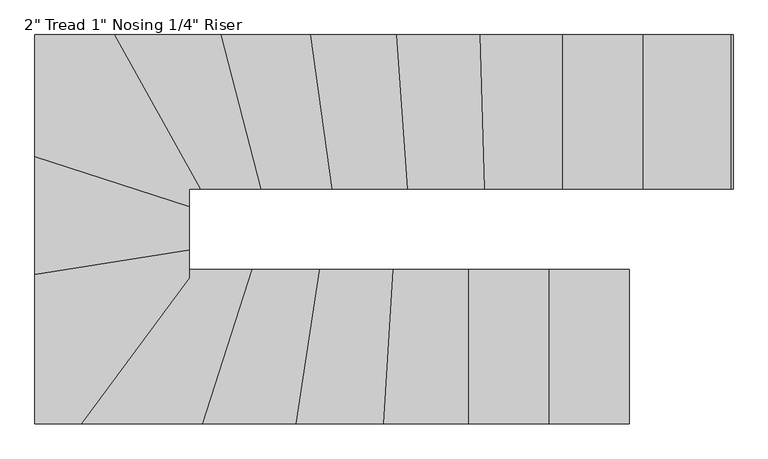
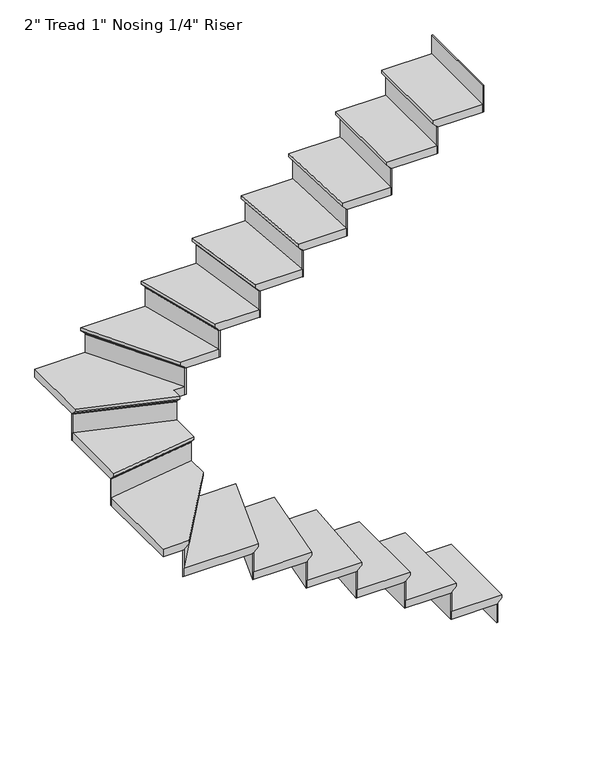
"""IFC4 building model written with IfcOpenShell, lengths in millimetres: stair flight geometry."""

from ifc_helpers import new_model, si_unit, origin, place, context, project, spatial, faceted_brep, source, transform, mapped, element, save


def stair_flight_19b8669d(model_context):
    return source(origin(), model_context, "Body", "Brep", [
        faceted_brep([(-264.8831579, 264.4433073, 9751.4833333), (-264.8831579, 264.4433073, 9770.5333333), (-264.8831579, -271.8029286, 9770.5333333), (-264.8831579, -271.8029286, 9751.4833333), (-290.2831579, 264.4433073, 9726.0833333), (-290.2831579, -271.8029286, 9726.0833333), (-569.6831579, 264.4433073, 9770.5333333), (-569.6831579, -271.8029286, 9770.5333333), (-290.2831579, -271.8029286, 9719.7333333), (-569.6831579, -271.8029286, 9719.7333333), (-569.6831579, 264.4433073, 9719.7333333), (-290.2831579, 264.4433073, 9719.7333333)], [[[0, 1, 2, 3]], [[4, 0, 3, 5]], [[2, 1, 6, 7]], [[8, 9, 10, 11]], [[2, 7, 9, 8, 5, 3]], [[8, 11, 4, 5]], [[6, 1, 0, 4, 11, 10]], [[7, 6, 10, 9]]]),
        faceted_brep([(-290.2831579, 264.4433073, 9719.7333333), (-290.2831579, 264.4433073, 9601.2), (-296.6331579, 264.4433073, 9601.2), (-296.6331579, 264.4433073, 9719.7333333), (-290.2831579, -271.8029286, 9719.7333333), (-296.6331579, -271.8029286, 9719.7333333), (-296.6331579, -271.8029286, 9601.2), (-290.2831579, -271.8029286, 9601.2)], [[[0, 1, 2, 3]], [[4, 5, 6, 7]], [[1, 0, 4, 7]], [[2, 1, 7, 6]], [[3, 2, 6, 5]], [[0, 3, 5, 4]]]),
        faceted_brep([(-569.6831579, 264.4433073, 9889.0666667), (-569.6831579, 264.4433073, 9719.7333333), (-576.0331579, 264.4433073, 9719.7333333), (-576.0331579, 264.4433073, 9889.0666667), (-569.6831579, -271.8029286, 9889.0666667), (-576.0331579, -271.8029286, 9889.0666667), (-576.0331579, -271.8029286, 9719.7333333), (-569.6831579, -271.8029286, 9719.7333333)], [[[0, 1, 2, 3]], [[4, 5, 6, 7]], [[1, 0, 4, 7]], [[2, 1, 7, 6]], [[3, 2, 6, 5]], [[0, 3, 5, 4]]]),
        faceted_brep([(-544.2831579, -271.8029286, 9939.8666667), (-544.2831579, 264.4433073, 9939.8666667), (-849.0831579, 264.4433073, 9939.8666667), (-849.0831579, -271.8029286, 9939.8666667), (-569.6831579, -271.8029286, 9889.0666667), (-849.0831579, -271.8029286, 9889.0666667), (-849.0831579, 264.4433073, 9889.0666667), (-569.6831579, 264.4433073, 9889.0666667), (-569.6831579, -271.8029286, 9895.4166667), (-544.2831579, -271.8029286, 9920.8166667), (-569.6831579, 264.4433073, 9895.4166667), (-544.2831579, 264.4433073, 9920.8166667)], [[[0, 1, 2, 3]], [[4, 5, 6, 7]], [[0, 3, 5, 4, 8, 9]], [[4, 7, 10, 8]], [[2, 1, 11, 10, 7, 6]], [[3, 2, 6, 5]], [[11, 1, 0, 9]], [[10, 11, 9, 8]]]),
        faceted_brep([(-849.0831579, 264.4433073, 10058.4), (-849.0831579, 264.4433073, 9889.0666667), (-855.4331579, 264.4433073, 9889.0666667), (-855.4331579, 264.4433073, 10058.4), (-849.0831579, -271.8029286, 10058.4), (-855.4331579, -271.8029286, 10058.4), (-855.4331579, -271.8029286, 9889.0666667), (-849.0831579, -271.8029286, 9889.0666667)], [[[0, 1, 2, 3]], [[4, 5, 6, 7]], [[1, 0, 4, 7]], [[2, 1, 7, 6]], [[3, 2, 6, 5]], [[0, 3, 5, 4]]]),
        faceted_brep([(-823.6831579, -271.8029286, 10109.2), (-823.6831579, 264.4433073, 10109.2), (-1112.6009003, 264.4433073, 10109.2), (-1144.4549627, -271.8029286, 10109.2), (-849.0831579, -271.8029286, 10058.4), (-1144.4549627, -271.8029286, 10058.4), (-1112.6009003, 264.4433073, 10058.4), (-849.0831579, 264.4433073, 10058.4), (-849.0831579, -271.8029286, 10064.75), (-823.6831579, -271.8029286, 10090.15), (-849.0831579, 264.4433073, 10064.75), (-823.6831579, 264.4433073, 10090.15)], [[[0, 1, 2, 3]], [[4, 5, 6, 7]], [[0, 3, 5, 4, 8, 9]], [[4, 7, 10, 8]], [[2, 1, 11, 10, 7, 6]], [[3, 2, 6, 5]], [[11, 1, 0, 9]], [[10, 11, 9, 8]]]),
        faceted_brep([(-1112.6009003, 264.4433073, 10227.7333333), (-1112.6009003, 264.4433073, 10058.4), (-1118.9620938, 264.4433073, 10058.4), (-1118.9620938, 264.4433073, 10227.7333333), (-1144.4549627, -271.8029286, 10227.7333333), (-1150.8161561, -271.8029286, 10227.7333333), (-1150.8161561, -271.8029286, 10058.4), (-1144.4549627, -271.8029286, 10058.4)], [[[0, 1, 2, 3]], [[4, 5, 6, 7]], [[1, 0, 4, 7]], [[2, 1, 7, 6]], [[3, 2, 6, 5]], [[0, 3, 5, 4]]]),
        faceted_brep([(-1119.0101891, -271.8029286, 10278.5333333), (-1087.1561267, 264.4433073, 10278.5333333), (-1367.1376579, 264.4433073, 10278.5333333), (-1449.2203373, -271.8029286, 10278.5333333), (-1144.4549627, -271.8029286, 10227.7333333), (-1449.2203373, -271.8029286, 10227.7333333), (-1367.1376579, 264.4433073, 10227.7333333), (-1112.6009003, 264.4433073, 10227.7333333), (-1144.4549627, -271.8029286, 10234.0833333), (-1119.0101891, -271.8029286, 10259.4833333), (-1112.6009003, 264.4433073, 10234.0833333), (-1087.1561267, 264.4433073, 10259.4833333)], [[[0, 1, 2, 3]], [[4, 5, 6, 7]], [[0, 3, 5, 4, 8, 9]], [[4, 7, 10, 8]], [[2, 1, 11, 10, 7, 6]], [[3, 2, 6, 5]], [[11, 1, 0, 9]], [[10, 11, 9, 8]]]),
        faceted_brep([(-1367.1376579, 264.4433073, 10397.0666667), (-1367.1376579, 264.4433073, 10227.7333333), (-1373.5616178, 264.4433073, 10227.7333333), (-1373.5616178, 264.4433073, 10397.0666667), (-1449.2203373, -271.8029286, 10397.0666667), (-1455.6442972, -271.8029286, 10397.0666667), (-1455.6442972, -271.8029286, 10227.7333333), (-1449.2203373, -271.8029286, 10227.7333333)], [[[0, 1, 2, 3]], [[4, 5, 6, 7]], [[1, 0, 4, 7]], [[2, 1, 7, 6]], [[3, 2, 6, 5]], [[0, 3, 5, 4]]]),
        faceted_brep([(-1423.5244976, -271.8029286, 10447.8666667), (-1341.4418182, 264.4433073, 10447.8666667), (-1602.0584075, 264.4433073, 10447.8666667), (-1775.0869242, -271.8029286, 10447.8666667), (-1449.2203373, -271.8029286, 10397.0666667), (-1775.0869242, -271.8029286, 10397.0666667), (-1602.0584075, 264.4433073, 10397.0666667), (-1367.1376579, 264.4433073, 10397.0666667), (-1449.2203373, -271.8029286, 10403.4166667), (-1423.5244976, -271.8029286, 10428.8166667), (-1367.1376579, 264.4433073, 10403.4166667), (-1341.4418182, 264.4433073, 10428.8166667)], [[[0, 1, 2, 3]], [[4, 5, 6, 7]], [[0, 3, 5, 4, 8, 9]], [[4, 7, 10, 8]], [[2, 1, 11, 10, 7, 6]], [[3, 2, 6, 5]], [[11, 1, 0, 9]], [[10, 11, 9, 8]]]),
        faceted_brep([(-1602.0584075, 264.4433073, 10566.4), (-1602.0584075, 264.4433073, 10397.0666667), (-1608.7307845, 264.4433073, 10397.0666667), (-1608.7307845, 264.4433073, 10566.4), (-1775.0869242, -271.8029286, 10566.4), (-1781.7593012, -271.8029286, 10566.4), (-1781.7593012, -271.8029286, 10397.0666667), (-1775.0869242, -271.8029286, 10397.0666667)], [[[0, 1, 2, 3]], [[4, 5, 6, 7]], [[1, 0, 4, 7]], [[2, 1, 7, 6]], [[3, 2, 6, 5]], [[0, 3, 5, 4]]]),
        faceted_brep([(-1748.3974163, -271.8029286, 10617.2), (-1575.3688995, 264.4433073, 10617.2), (-1792.6148498, 264.4433073, 10617.2), (-1792.6148498, 277.721026, 10617.2), (-2200.2950016, -271.8029286, 10617.2), (-1775.0869242, -271.8029286, 10566.4), (-2200.2950016, -271.8029286, 10566.4), (-1792.6148498, 277.721026, 10566.4), (-1792.6148498, 264.4433073, 10566.4), (-1602.0584075, 264.4433073, 10566.4), (-1775.0869242, -271.8029286, 10572.75), (-1748.3974163, -271.8029286, 10598.15), (-1602.0584075, 264.4433073, 10572.75), (-1575.3688995, 264.4433073, 10598.15)], [[[0, 1, 2, 3, 4]], [[5, 6, 7, 8, 9]], [[0, 4, 6, 5, 10, 11]], [[5, 9, 12, 10]], [[2, 1, 13, 12, 9, 8]], [[4, 3, 7, 6]], [[13, 1, 0, 11]], [[12, 13, 11, 10]], [[3, 2, 8, 7]]]),
        faceted_brep([(-1792.6148498, 277.721026, 10735.7333333), (-1792.6148498, 277.721026, 10566.4), (-1792.6148498, 288.3786511, 10566.4), (-1792.6148498, 288.3786511, 10735.7333333), (-2200.2950016, -271.8029286, 10735.7333333), (-2208.2016673, -271.8029286, 10735.7333333), (-2208.2016673, -271.8029286, 10566.4), (-2200.2950016, -271.8029286, 10566.4)], [[[0, 1, 2, 3]], [[4, 5, 6, 7]], [[1, 0, 4, 7]], [[2, 1, 7, 6]], [[3, 2, 6, 5]], [[0, 3, 5, 4]]]),
        faceted_brep([(-2328.8610857, 272.9225747, 10786.5333333), (-2328.8610857, -271.8029286, 10786.5333333), (-2168.6683387, -271.8029286, 10786.5333333), (-1792.6148498, 235.0905257, 10786.5333333), (-1792.6148498, 358.7948785, 10786.5333333), (-2328.8610857, -271.8029286, 10735.7333333), (-2328.8610857, 272.9225747, 10735.7333333), (-1792.6148498, 358.7948785, 10735.7333333), (-1792.6148498, 277.721026, 10735.7333333), (-2200.2950016, -271.8029286, 10735.7333333), (-2200.2950016, -271.8029286, 10742.0833333), (-2168.6683387, -271.8029286, 10767.4833333), (-1792.6148498, 277.721026, 10742.0833333), (-1792.6148498, 235.0905257, 10767.4833333)], [[[0, 1, 2, 3, 4]], [[5, 6, 7, 8, 9]], [[1, 0, 6, 5]], [[2, 1, 5, 9, 10, 11]], [[9, 8, 12, 10]], [[4, 3, 13, 12, 8, 7]], [[0, 4, 7, 6]], [[13, 3, 2, 11]], [[12, 13, 11, 10]]]),
        faceted_brep([(-1792.6148498, 358.7948785, 10905.0666667), (-1792.6148498, 358.7948785, 10735.7333333), (-1792.6148498, 365.2257813, 10735.7333333), (-1792.6148498, 365.2257813, 10905.0666667), (-2328.8610857, 272.9225747, 10905.0666667), (-2328.8610857, 279.3534775, 10905.0666667), (-2328.8610857, 279.3534775, 10735.7333333), (-2328.8610857, 272.9225747, 10735.7333333)], [[[0, 1, 2, 3]], [[4, 5, 6, 7]], [[1, 0, 4, 7]], [[2, 1, 7, 6]], [[3, 2, 6, 5]], [[0, 3, 5, 4]]]),
        faceted_brep([(-2328.8610857, 247.1989634, 10955.8666667), (-1792.6148498, 333.0712672, 10955.8666667), (-1792.6148498, 510.0383883, 10955.8666667), (-2328.8610857, 683.2061106, 10955.8666667), (-2328.8610857, 272.9225747, 10905.0666667), (-2328.8610857, 683.2061106, 10905.0666667), (-1792.6148498, 510.0383883, 10905.0666667), (-1792.6148498, 358.7948785, 10905.0666667), (-2328.8610857, 272.9225747, 10911.4166667), (-2328.8610857, 247.1989634, 10936.8166667), (-1792.6148498, 358.7948785, 10911.4166667), (-1792.6148498, 333.0712672, 10936.8166667)], [[[0, 1, 2, 3]], [[4, 5, 6, 7]], [[0, 3, 5, 4, 8, 9]], [[4, 7, 10, 8]], [[3, 2, 6, 5]], [[11, 1, 0, 9]], [[10, 11, 9, 8]], [[2, 1, 11, 10, 7, 6]]]),
        faceted_brep([(-1792.6148498, 510.0383883, 11074.4), (-1792.6148498, 510.0383883, 10905.0666667), (-1792.6148498, 516.7112716, 10905.0666667), (-1792.6148498, 516.7112716, 11074.4), (-2328.8610857, 683.2061106, 11074.4), (-2328.8610857, 689.878994, 11074.4), (-2328.8610857, 689.878994, 10905.0666667), (-2328.8610857, 683.2061106, 10905.0666667)], [[[0, 1, 2, 3]], [[4, 5, 6, 7]], [[1, 0, 4, 7]], [[2, 1, 7, 6]], [[3, 2, 6, 5]], [[0, 3, 5, 4]]]),
        faceted_brep([(-2021.9568272, 1080.0895433, 11125.2), (-2328.8610857, 1080.0895433, 11125.2), (-2328.8610857, 656.5145772, 11125.2), (-1792.6148498, 483.3468548, 11125.2), (-1792.6148498, 543.8433073, 11125.2), (-1724.5287393, 543.8433073, 11125.2), (-2328.8610857, 1080.0895433, 11074.4), (-2021.9568272, 1080.0895433, 11074.4), (-1724.5287393, 543.8433073, 11074.4), (-1792.6148498, 543.8433073, 11074.4), (-1792.6148498, 510.0383883, 11074.4), (-2328.8610857, 683.2061106, 11074.4), (-1792.6148498, 510.0383883, 11080.75), (-2328.8610857, 683.2061106, 11080.75), (-1792.6148498, 483.3468548, 11106.15), (-2328.8610857, 656.5145772, 11106.15)], [[[0, 1, 2, 3, 4, 5]], [[6, 7, 8, 9, 10, 11]], [[1, 0, 7, 6]], [[11, 10, 12, 13]], [[4, 3, 14, 12, 10, 9]], [[0, 5, 8, 7]], [[14, 3, 2, 15]], [[12, 14, 15, 13]], [[2, 1, 6, 11, 13, 15]], [[5, 4, 9, 8]]]),
        faceted_brep([(-1724.5287393, 543.8433073, 11243.7333333), (-1724.5287393, 543.8433073, 11074.4), (-1717.2673962, 543.8433073, 11074.4), (-1717.2673962, 543.8433073, 11243.7333333), (-2021.9568272, 1080.0895433, 11243.7333333), (-2014.6954841, 1080.0895433, 11243.7333333), (-2014.6954841, 1080.0895433, 11074.4), (-2021.9568272, 1080.0895433, 11074.4)], [[[0, 1, 2, 3]], [[4, 5, 6, 7]], [[1, 0, 4, 7]], [[2, 1, 7, 6]], [[3, 2, 6, 5]], [[0, 3, 5, 4]]]),
        faceted_brep([(-2051.0021996, 1080.0895433, 11294.5333333), (-1753.5741117, 543.8433073, 11294.5333333), (-1517.487325, 543.8433073, 11294.5333333), (-1656.0375972, 1080.0895433, 11294.5333333), (-2021.9568272, 1080.0895433, 11243.7333333), (-1656.0375972, 1080.0895433, 11243.7333333), (-1517.487325, 543.8433073, 11243.7333333), (-1724.5287393, 543.8433073, 11243.7333333), (-2021.9568272, 1080.0895433, 11250.0833333), (-2051.0021996, 1080.0895433, 11275.4833333), (-1724.5287393, 543.8433073, 11250.0833333), (-1753.5741117, 543.8433073, 11275.4833333)], [[[0, 1, 2, 3]], [[4, 5, 6, 7]], [[0, 3, 5, 4, 8, 9]], [[4, 7, 10, 8]], [[2, 1, 11, 10, 7, 6]], [[3, 2, 6, 5]], [[11, 1, 0, 9]], [[10, 11, 9, 8]]]),
        faceted_brep([(-1517.487325, 543.8433073, 11413.0666667), (-1517.487325, 543.8433073, 11243.7333333), (-1510.9288005, 543.8433073, 11243.7333333), (-1510.9288005, 543.8433073, 11413.0666667), (-1656.0375972, 1080.0895433, 11413.0666667), (-1649.4790727, 1080.0895433, 11413.0666667), (-1649.4790727, 1080.0895433, 11243.7333333), (-1656.0375972, 1080.0895433, 11243.7333333)], [[[0, 1, 2, 3]], [[4, 5, 6, 7]], [[1, 0, 4, 7]], [[2, 1, 7, 6]], [[3, 2, 6, 5]], [[0, 3, 5, 4]]]),
        faceted_brep([(-1682.2716952, 1080.0895433, 11463.8666667), (-1543.721423, 543.8433073, 11463.8666667), (-1271.2041837, 543.8433073, 11463.8666667), (-1344.713853, 1080.0895433, 11463.8666667), (-1656.0375972, 1080.0895433, 11413.0666667), (-1344.713853, 1080.0895433, 11413.0666667), (-1271.2041837, 543.8433073, 11413.0666667), (-1517.487325, 543.8433073, 11413.0666667), (-1656.0375972, 1080.0895433, 11419.4166667), (-1682.2716952, 1080.0895433, 11444.8166667), (-1517.487325, 543.8433073, 11419.4166667), (-1543.721423, 543.8433073, 11444.8166667)], [[[0, 1, 2, 3]], [[4, 5, 6, 7]], [[0, 3, 5, 4, 8, 9]], [[4, 7, 10, 8]], [[2, 1, 11, 10, 7, 6]], [[3, 2, 6, 5]], [[11, 1, 0, 9]], [[10, 11, 9, 8]]]),
        faceted_brep([(-1271.2041837, 543.8433073, 11582.4), (-1271.2041837, 543.8433073, 11413.0666667), (-1264.7947985, 543.8433073, 11413.0666667), (-1264.7947985, 543.8433073, 11582.4), (-1344.713853, 1080.0895433, 11582.4), (-1338.3044678, 1080.0895433, 11582.4), (-1338.3044678, 1080.0895433, 11413.0666667), (-1344.713853, 1080.0895433, 11413.0666667)], [[[0, 1, 2, 3]], [[4, 5, 6, 7]], [[1, 0, 4, 7]], [[2, 1, 7, 6]], [[3, 2, 6, 5]], [[0, 3, 5, 4]]]),
        faceted_brep([(-1370.3513937, 1080.0895433, 11633.2), (-1296.8417245, 543.8433073, 11633.2), (-1009.7763573, 543.8433073, 11633.2), (-1047.6899509, 1080.0895433, 11633.2), (-1344.713853, 1080.0895433, 11582.4), (-1047.6899509, 1080.0895433, 11582.4), (-1009.7763573, 543.8433073, 11582.4), (-1271.2041837, 543.8433073, 11582.4), (-1344.713853, 1080.0895433, 11588.75), (-1370.3513937, 1080.0895433, 11614.15), (-1271.2041837, 543.8433073, 11588.75), (-1296.8417245, 543.8433073, 11614.15)], [[[0, 1, 2, 3]], [[4, 5, 6, 7]], [[0, 3, 5, 4, 8, 9]], [[4, 7, 10, 8]], [[2, 1, 11, 10, 7, 6]], [[3, 2, 6, 5]], [[11, 1, 0, 9]], [[10, 11, 9, 8]]]),
        faceted_brep([(-1009.7763573, 543.8433073, 11751.7333333), (-1009.7763573, 543.8433073, 11582.4), (-1003.4105061, 543.8433073, 11582.4), (-1003.4105061, 543.8433073, 11751.7333333), (-1047.6899509, 1080.0895433, 11751.7333333), (-1041.3240997, 1080.0895433, 11751.7333333), (-1041.3240997, 1080.0895433, 11582.4), (-1047.6899509, 1080.0895433, 11582.4)], [[[0, 1, 2, 3]], [[4, 5, 6, 7]], [[1, 0, 4, 7]], [[2, 1, 7, 6]], [[3, 2, 6, 5]], [[0, 3, 5, 4]]]),
        faceted_brep([(-1073.1533559, 1080.0895433, 11802.5333333), (-1035.2397623, 543.8433073, 11802.5333333), (-741.6570892, 543.8433073, 11802.5333333), (-757.1149275, 1080.0895433, 11802.5333333), (-1047.6899509, 1080.0895433, 11751.7333333), (-757.1149275, 1080.0895433, 11751.7333333), (-741.6570892, 543.8433073, 11751.7333333), (-1009.7763573, 543.8433073, 11751.7333333), (-1047.6899509, 1080.0895433, 11758.0833333), (-1073.1533559, 1080.0895433, 11783.4833333), (-1009.7763573, 543.8433073, 11758.0833333), (-1035.2397623, 543.8433073, 11783.4833333)], [[[0, 1, 2, 3]], [[4, 5, 6, 7]], [[0, 3, 5, 4, 8, 9]], [[4, 7, 10, 8]], [[2, 1, 11, 10, 7, 6]], [[3, 2, 6, 5]], [[11, 1, 0, 9]], [[10, 11, 9, 8]]]),
        faceted_brep([(-741.6570892, 543.8433073, 11921.0666667), (-741.6570892, 543.8433073, 11751.7333333), (-735.3044516, 543.8433073, 11751.7333333), (-735.3044516, 543.8433073, 11921.0666667), (-757.1149275, 1080.0895433, 11921.0666667), (-750.7622898, 1080.0895433, 11921.0666667), (-750.7622898, 1080.0895433, 11751.7333333), (-757.1149275, 1080.0895433, 11751.7333333)], [[[0, 1, 2, 3]], [[4, 5, 6, 7]], [[1, 0, 4, 7]], [[2, 1, 7, 6]], [[3, 2, 6, 5]], [[0, 3, 5, 4]]]),
        faceted_brep([(-782.5254783, 1080.0895433, 11971.8666667), (-767.06764, 543.8433073, 11971.8666667), (-469.9965591, 543.8433073, 11971.8666667), (-469.9965591, 1080.0895433, 11971.8666667), (-757.1149275, 1080.0895433, 11921.0666667), (-469.9965591, 1080.0895433, 11921.0666667), (-469.9965591, 543.8433073, 11921.0666667), (-741.6570892, 543.8433073, 11921.0666667), (-757.1149275, 1080.0895433, 11927.4166667), (-782.5254783, 1080.0895433, 11952.8166667), (-741.6570892, 543.8433073, 11927.4166667), (-767.06764, 543.8433073, 11952.8166667)], [[[0, 1, 2, 3]], [[4, 5, 6, 7]], [[0, 3, 5, 4, 8, 9]], [[4, 7, 10, 8]], [[2, 1, 11, 10, 7, 6]], [[3, 2, 6, 5]], [[11, 1, 0, 9]], [[10, 11, 9, 8]]]),
        faceted_brep([(-469.9965591, 543.8433073, 12090.4), (-469.9965591, 543.8433073, 11921.0666667), (-463.6465591, 543.8433073, 11921.0666667), (-463.6465591, 543.8433073, 12090.4), (-469.9965591, 1080.0895433, 12090.4), (-463.6465591, 1080.0895433, 12090.4), (-463.6465591, 1080.0895433, 11921.0666667), (-469.9965591, 1080.0895433, 11921.0666667)], [[[0, 1, 2, 3]], [[4, 5, 6, 7]], [[1, 0, 4, 7]], [[2, 1, 7, 6]], [[3, 2, 6, 5]], [[0, 3, 5, 4]]]),
        faceted_brep([(-495.3965591, 1080.0895433, 12141.2), (-495.3965591, 543.8433073, 12141.2), (-190.5965591, 543.8433073, 12141.2), (-190.5965591, 1080.0895433, 12141.2), (-469.9965591, 1080.0895433, 12090.4), (-190.5965591, 1080.0895433, 12090.4), (-190.5965591, 543.8433073, 12090.4), (-469.9965591, 543.8433073, 12090.4), (-469.9965591, 1080.0895433, 12096.75), (-495.3965591, 1080.0895433, 12122.15), (-469.9965591, 543.8433073, 12096.75), (-495.3965591, 543.8433073, 12122.15)], [[[0, 1, 2, 3]], [[4, 5, 6, 7]], [[0, 3, 5, 4, 8, 9]], [[4, 7, 10, 8]], [[2, 1, 11, 10, 7, 6]], [[3, 2, 6, 5]], [[11, 1, 0, 9]], [[10, 11, 9, 8]]]),
        faceted_brep([(-190.5965591, 543.8433073, 12259.7333333), (-190.5965591, 543.8433073, 12090.4), (-184.2465591, 543.8433073, 12090.4), (-184.2465591, 543.8433073, 12259.7333333), (-190.5965591, 1080.0895433, 12259.7333333), (-184.2465591, 1080.0895433, 12259.7333333), (-184.2465591, 1080.0895433, 12090.4), (-190.5965591, 1080.0895433, 12090.4)], [[[0, 1, 2, 3]], [[4, 5, 6, 7]], [[1, 0, 4, 7]], [[2, 1, 7, 6]], [[3, 2, 6, 5]], [[0, 3, 5, 4]]]),
        faceted_brep([(88.8034409, 543.8433073, 12429.0666667), (88.8034409, 543.8433073, 12259.7333333), (95.1534409, 543.8433073, 12259.7333333), (95.1534409, 543.8433073, 12429.0666667), (88.8034409, 1080.0895433, 12429.0666667), (95.1534409, 1080.0895433, 12429.0666667), (95.1534409, 1080.0895433, 12259.7333333), (88.8034409, 1080.0895433, 12259.7333333)], [[[0, 1, 2, 3]], [[4, 5, 6, 7]], [[1, 0, 4, 7]], [[2, 1, 7, 6]], [[3, 2, 6, 5]], [[0, 3, 5, 4]]]),
        faceted_brep([(-215.9965591, 1080.0895433, 12310.5333333), (-215.9965591, 543.8433073, 12310.5333333), (88.8034409, 543.8433073, 12310.5333333), (88.8034409, 1080.0895433, 12310.5333333), (-190.5965591, 1080.0895433, 12259.7333333), (88.8034409, 1080.0895433, 12259.7333333), (88.8034409, 543.8433073, 12259.7333333), (-190.5965591, 543.8433073, 12259.7333333), (-190.5965591, 1080.0895433, 12266.0833333), (-215.9965591, 1080.0895433, 12291.4833333), (-190.5965591, 543.8433073, 12266.0833333), (-215.9965591, 543.8433073, 12291.4833333)], [[[0, 1, 2, 3]], [[4, 5, 6, 7]], [[0, 3, 5, 4, 8, 9]], [[4, 7, 10, 8]], [[2, 1, 11, 10, 7, 6]], [[3, 2, 6, 5]], [[11, 1, 0, 9]], [[10, 11, 9, 8]]]),
    ])


if __name__ == "__main__":
    model = new_model("IFC4")
    model_context = context("Model", 3, world=origin())
    ifc_project = project(units=[si_unit("LENGTHUNIT", "METRE", prefix="MILLI")], contexts=[model_context])
    site = spatial("IfcSite", under=ifc_project)
    building = spatial("IfcBuilding", under=site)
    placement = place(None, origin())
    stair_flight_shape = stair_flight_19b8669d(model_context)
    element("IfcStairFlight", 1, ObjectType="2\" Tread 1\" Nosing 1/4\" Riser", at=placement, inside=building, context=model_context, shape_type="MappedRepresentation", body=[
        mapped(stair_flight_shape, transform((0.0, 0.0, 0.0), x_axis=(1.0, 0.0, 0.0), y_axis=(0.0, 1.0, 0.0), z_axis=(0.0, 0.0, 1.0))),
    ])
    save(model, "model.ifc")
